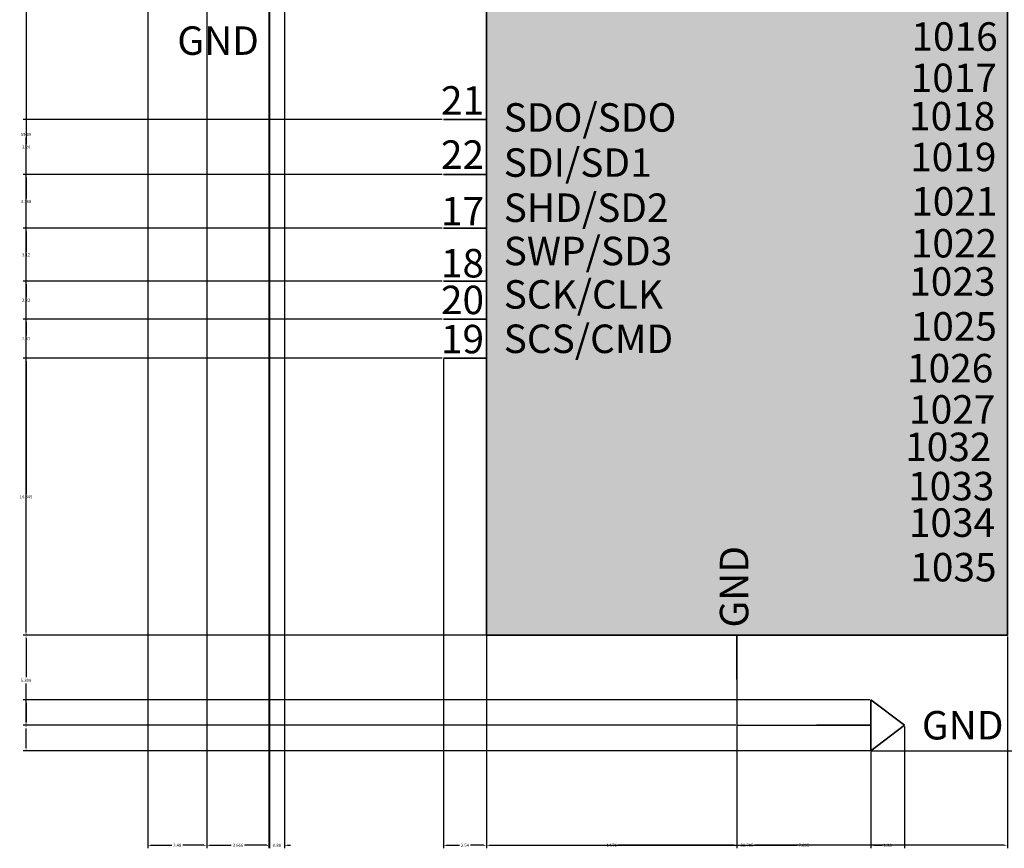
# Model space of a CAD drawing. Units: inches. Extents: x 23 to 132, y 5 to 105.
# Tile 1 of 14: x 23 to 81, y 5 to 54. Entities that reach past the tile are written whole.
import ezdxf

# ---------------------------------------------------------------- set-up
doc = ezdxf.new("R2010")
doc.units = ezdxf.units.IN
doc.header["$MEASUREMENT"] = 0
for name, color, linetype, lineweight in [('A-ANNO-DIMS', 2, 'Continuous', 18), ('E-ANNO-IDEN', 4, 'Continuous', 18), ('E-ANNO-TEXT', 3, 'Continuous', 18), ('E-SYMB', 1, 'Continuous', 35), ('E-SYMB-PATT', 1, 'Continuous', 18), ('E-WIRE', 3, 'Continuous', 25)]:
    doc.layers.add(name, color=color, linetype=linetype, lineweight=lineweight)
doc.styles.get("Standard").update_dxf_attribs({"font": 'arial.ttf'})
doc.dimstyles.get("Standard").update_dxf_attribs({"dimtxt": 0.18, "dimasz": 0.18, "dimexe": 0.18, "dimexo": 0.0625, "dimgap": 0.09, "dimtad": 0, "dimtih": 1, "dimtoh": 1, "dimdec": 4, "dimzin": 0, "dimdsep": 46, "dimtxsty": 'Standard', "dimcen": 0.09, "dimadec": 0, "dimazin": 0, "dimtfac": 1, "dimtdec": 4, "dimtofl": 0, "dimtmove": 0, "dimatfit": 3, "dimfxl": 1, "dimtolj": 1, "dimtzin": 0, "dimarcsym": 0})

# ---------------------------------------------------------------- blocks, each defined once
blk = doc.blocks.new('*D3')
at = {"layer": 'A-ANNO-DIMS', "color": 0, "lineweight": -2, "transparency": 16777216}
for p, q in [((121.409, 99.285), (129.239, 99.285)), ((129.059, 99.105), (129.059, 55.423)), ((129.059, 11.378), (129.059, 55.06)), ((72.981, 11.198), (129.239, 11.198))]:
    blk.add_line(p, q, dxfattribs=at)
at = {"layer": 'A-ANNO-DIMS', "color": 0, "transparency": 16777216}
for points in [[(129.029, 99.105), (129.089, 99.105), (129.059, 99.285)], [(129.029, 11.378), (129.089, 11.378), (129.059, 11.198)]]:
    blk.add_solid(points, dxfattribs=at)
at = {"layer": 'Defpoints', "color": 0, "transparency": 16777216}
for p in [(121.346, 99.285), (129.059, 99.285), (72.919, 11.198)]:
    blk.add_point(p, dxfattribs=at)
at = {"layer": 'A-ANNO-DIMS', "color": 0, "transparency": 16777216, "insert": (129.059, 55.241), "char_height": 0.18, "attachment_point": 5}
blk.add_mtext('\\A1;88.09', dxfattribs=at)
blk = doc.blocks.new('*D4')
at = {"layer": 'A-ANNO-DIMS', "color": 0, "lineweight": -2, "transparency": 16777216}
for p, q in [((50.265, 17.944), (50.265, 5.443)), ((80.969, 17.944), (80.969, 5.443)), ((50.445, 5.623), (65.153, 5.623)), ((80.789, 5.623), (66.081, 5.623))]:
    blk.add_line(p, q, dxfattribs=at)
at = {"layer": 'A-ANNO-DIMS', "color": 0, "transparency": 16777216}
for points in [[(50.445, 5.653), (50.445, 5.593), (50.265, 5.623)], [(80.789, 5.653), (80.789, 5.593), (80.969, 5.623)]]:
    blk.add_solid(points, dxfattribs=at)
at = {"layer": 'Defpoints', "color": 0, "transparency": 16777216}
for p in [(50.265, 18.007), (80.969, 18.007), (80.969, 5.623)]:
    blk.add_point(p, dxfattribs=at)
at = {"layer": 'A-ANNO-DIMS', "color": 0, "transparency": 16777216, "insert": (65.617, 5.623), "char_height": 0.18, "attachment_point": 5}
blk.add_mtext('\\A1;30.705', dxfattribs=at)
blk = doc.blocks.new('*D5')
at = {"layer": 'A-ANNO-DIMS', "color": 0, "lineweight": -2, "transparency": 16777216}
for p, q in [((50.265, 17.944), (50.265, 5.443)), ((65.024, 17.944), (65.024, 5.443)), ((50.445, 5.623), (57.259, 5.623)), ((64.844, 5.623), (58.029, 5.623))]:
    blk.add_line(p, q, dxfattribs=at)
at = {"layer": 'A-ANNO-DIMS', "color": 0, "transparency": 16777216}
for points in [[(50.445, 5.653), (50.445, 5.593), (50.265, 5.623)], [(64.844, 5.653), (64.844, 5.593), (65.024, 5.623)]]:
    blk.add_solid(points, dxfattribs=at)
at = {"layer": 'Defpoints', "color": 0, "transparency": 16777216}
for p in [(50.265, 18.007), (65.024, 18.007), (65.024, 5.623)]:
    blk.add_point(p, dxfattribs=at)
at = {"layer": 'A-ANNO-DIMS', "color": 0, "transparency": 16777216, "insert": (57.644, 5.623), "char_height": 0.18, "attachment_point": 5}
blk.add_mtext('\\A1;14.76', dxfattribs=at)
blk = doc.blocks.new('*D6')
at = {"layer": 'A-ANNO-DIMS', "color": 0, "lineweight": -2, "transparency": 16777216}
for p, q in [((50.202, 77.095), (22.942, 77.095)), ((23.122, 76.915), (23.122, 47.733)), ((23.122, 18.187), (23.122, 47.369)), ((50.202, 18.007), (22.942, 18.007))]:
    blk.add_line(p, q, dxfattribs=at)
at = {"layer": 'A-ANNO-DIMS', "color": 0, "transparency": 16777216}
for points in [[(23.092, 76.915), (23.152, 76.915), (23.122, 77.095)], [(23.092, 18.187), (23.152, 18.187), (23.122, 18.007)]]:
    blk.add_solid(points, dxfattribs=at)
at = {"layer": 'Defpoints', "color": 0, "transparency": 16777216}
for p in [(23.122, 77.095), (50.265, 77.095), (50.265, 18.007)]:
    blk.add_point(p, dxfattribs=at)
at = {"layer": 'A-ANNO-DIMS', "color": 0, "transparency": 16777216, "insert": (23.122, 47.551), "char_height": 0.18, "attachment_point": 5}
blk.add_mtext('\\A1;59.09', dxfattribs=at)
blk = doc.blocks.new('*D8')
at = {"layer": 'A-ANNO-DIMS', "color": 0, "lineweight": -2, "transparency": 16777216}
for p, q in [((64.961, 18.007), (22.942, 18.007)), ((23.122, 17.827), (23.122, 15.534)), ((23.122, 12.878), (23.122, 15.17)), ((64.961, 12.698), (22.942, 12.698))]:
    blk.add_line(p, q, dxfattribs=at)
at = {"layer": 'A-ANNO-DIMS', "color": 0, "transparency": 16777216}
for points in [[(23.092, 17.827), (23.152, 17.827), (23.122, 18.007)], [(23.092, 12.878), (23.152, 12.878), (23.122, 12.698)]]:
    blk.add_solid(points, dxfattribs=at)
at = {"layer": 'Defpoints', "color": 0, "transparency": 16777216}
for p in [(23.122, 18.007), (65.024, 18.007), (65.024, 12.698)]:
    blk.add_point(p, dxfattribs=at)
at = {"layer": 'A-ANNO-DIMS', "color": 0, "transparency": 16777216, "insert": (23.122, 15.352), "char_height": 0.18, "attachment_point": 5}
blk.add_mtext('\\A1;5.308', dxfattribs=at)
blk = doc.blocks.new('*D9')
at = {"layer": 'A-ANNO-DIMS', "color": 0, "lineweight": -2, "transparency": 16777216}
for p, q in [((65.024, 12.636), (65.024, 5.443)), ((72.919, 12.636), (72.919, 5.443)), ((65.204, 5.623), (68.578, 5.623)), ((72.739, 5.623), (69.365, 5.623))]:
    blk.add_line(p, q, dxfattribs=at)
at = {"layer": 'A-ANNO-DIMS', "color": 0, "transparency": 16777216}
for points in [[(65.204, 5.653), (65.204, 5.593), (65.024, 5.623)], [(72.739, 5.653), (72.739, 5.593), (72.919, 5.623)]]:
    blk.add_solid(points, dxfattribs=at)
at = {"layer": 'Defpoints', "color": 0, "transparency": 16777216}
for p in [(65.024, 12.698), (72.919, 12.698), (72.919, 5.623)]:
    blk.add_point(p, dxfattribs=at)
at = {"layer": 'A-ANNO-DIMS', "color": 0, "transparency": 16777216, "insert": (68.971, 5.623), "char_height": 0.18, "attachment_point": 5}
blk.add_mtext('\\A1;7.895', dxfattribs=at)
blk = doc.blocks.new('*D10')
at = {"layer": 'A-ANNO-DIMS', "color": 0, "lineweight": -2, "transparency": 16777216}
for p, q in [((74.903, 12.636), (74.903, 5.443)), ((72.919, 11.136), (72.919, 5.443)), ((73.099, 5.623), (73.595, 5.623)), ((74.723, 5.623), (74.226, 5.623))]:
    blk.add_line(p, q, dxfattribs=at)
at = {"layer": 'A-ANNO-DIMS', "color": 0, "transparency": 16777216}
for points in [[(73.099, 5.653), (73.099, 5.593), (72.919, 5.623)], [(74.723, 5.653), (74.723, 5.593), (74.903, 5.623)]]:
    blk.add_solid(points, dxfattribs=at)
at = {"layer": 'Defpoints', "color": 0, "transparency": 16777216}
for p in [(74.903, 12.698), (72.919, 11.198), (74.903, 5.623)]:
    blk.add_point(p, dxfattribs=at)
at = {"layer": 'A-ANNO-DIMS', "color": 0, "transparency": 16777216, "insert": (73.911, 5.623), "char_height": 0.18, "attachment_point": 5}
blk.add_mtext('\\A1;1.98', dxfattribs=at)
blk = doc.blocks.new('*D11')
at = {"layer": 'A-ANNO-DIMS', "color": 0, "lineweight": -2, "transparency": 16777216}
for p, q in [((72.856, 14.198), (22.942, 14.198)), ((23.122, 14.018), (23.122, 12.88)), ((23.122, 11.378), (23.122, 12.516)), ((72.856, 11.198), (22.942, 11.198))]:
    blk.add_line(p, q, dxfattribs=at)
at = {"layer": 'A-ANNO-DIMS', "color": 0, "transparency": 16777216}
for points in [[(23.092, 14.018), (23.152, 14.018), (23.122, 14.198)], [(23.092, 11.378), (23.152, 11.378), (23.122, 11.198)]]:
    blk.add_solid(points, dxfattribs=at)
at = {"layer": 'Defpoints', "color": 0, "transparency": 16777216}
for p in [(23.122, 14.198), (72.919, 14.198), (72.919, 11.198)]:
    blk.add_point(p, dxfattribs=at)
at = {"layer": 'A-ANNO-DIMS', "color": 0, "transparency": 16777216, "insert": (23.122, 12.698), "char_height": 0.18, "attachment_point": 5}
blk.add_mtext('\\A1;3', dxfattribs=at)
blk = doc.blocks.new('*D13')
at = {"layer": 'A-ANNO-DIMS', "color": 0, "lineweight": -2, "transparency": 16777216}
for p, q in [((47.72, 34.289), (47.72, 5.443)), ((50.265, 34.289), (50.265, 5.443)), ((47.9, 5.623), (48.667, 5.623)), ((50.085, 5.623), (49.317, 5.623))]:
    blk.add_line(p, q, dxfattribs=at)
at = {"layer": 'A-ANNO-DIMS', "color": 0, "transparency": 16777216}
for points in [[(47.9, 5.653), (47.9, 5.593), (47.72, 5.623)], [(50.085, 5.653), (50.085, 5.593), (50.265, 5.623)]]:
    blk.add_solid(points, dxfattribs=at)
at = {"layer": 'Defpoints', "color": 0, "transparency": 16777216}
for p in [(47.72, 34.351), (50.265, 34.351), (50.265, 5.623)]:
    blk.add_point(p, dxfattribs=at)
at = {"layer": 'A-ANNO-DIMS', "color": 0, "transparency": 16777216, "insert": (48.992, 5.623), "char_height": 0.18, "attachment_point": 5}
blk.add_mtext('\\A1;2.54', dxfattribs=at)
blk = doc.blocks.new('*D18')
at = {"layer": 'A-ANNO-DIMS', "color": 0, "lineweight": -2, "transparency": 16777216}
for p, q in [((47.658, 34.351), (22.942, 34.351)), ((23.122, 34.171), (23.122, 26.361)), ((23.122, 18.187), (23.122, 25.997)), ((50.202, 18.007), (22.942, 18.007))]:
    blk.add_line(p, q, dxfattribs=at)
at = {"layer": 'A-ANNO-DIMS', "color": 0, "transparency": 16777216}
for points in [[(23.092, 34.171), (23.152, 34.171), (23.122, 34.351)], [(23.092, 18.187), (23.152, 18.187), (23.122, 18.007)]]:
    blk.add_solid(points, dxfattribs=at)
at = {"layer": 'Defpoints', "color": 0, "transparency": 16777216}
for p in [(23.122, 34.351), (47.72, 34.351), (50.265, 18.007)]:
    blk.add_point(p, dxfattribs=at)
at = {"layer": 'A-ANNO-DIMS', "color": 0, "transparency": 16777216, "insert": (23.122, 26.179), "char_height": 0.18, "attachment_point": 5}
blk.add_mtext('\\A1;16.345', dxfattribs=at)
blk = doc.blocks.new('*D19')
at = {"layer": 'A-ANNO-DIMS', "color": 0, "lineweight": -2, "transparency": 16777216}
for p, q in [((47.658, 36.662), (22.942, 36.662)), ((23.122, 36.482), (23.122, 35.688)), ((23.122, 34.531), (23.122, 35.325)), ((47.658, 34.351), (22.942, 34.351))]:
    blk.add_line(p, q, dxfattribs=at)
at = {"layer": 'A-ANNO-DIMS', "color": 0, "transparency": 16777216}
for points in [[(23.092, 36.482), (23.152, 36.482), (23.122, 36.662)], [(23.092, 34.531), (23.152, 34.531), (23.122, 34.351)]]:
    blk.add_solid(points, dxfattribs=at)
at = {"layer": 'Defpoints', "color": 0, "transparency": 16777216}
for p in [(23.122, 36.662), (47.72, 36.662), (47.72, 34.351)]:
    blk.add_point(p, dxfattribs=at)
at = {"layer": 'A-ANNO-DIMS', "color": 0, "transparency": 16777216, "insert": (23.122, 35.506), "char_height": 0.18, "attachment_point": 5}
blk.add_mtext('\\A1;2.31', dxfattribs=at)
blk = doc.blocks.new('*D20')
at = {"layer": 'A-ANNO-DIMS', "color": 0, "lineweight": -2, "transparency": 16777216}
for p, q in [((47.658, 38.89), (22.942, 38.89)), ((23.122, 38.71), (23.122, 37.958)), ((23.122, 36.842), (23.122, 37.594)), ((47.658, 36.662), (22.942, 36.662))]:
    blk.add_line(p, q, dxfattribs=at)
at = {"layer": 'A-ANNO-DIMS', "color": 0, "transparency": 16777216}
for points in [[(23.092, 38.71), (23.152, 38.71), (23.122, 38.89)], [(23.092, 36.842), (23.152, 36.842), (23.122, 36.662)]]:
    blk.add_solid(points, dxfattribs=at)
at = {"layer": 'Defpoints', "color": 0, "transparency": 16777216}
for p in [(23.122, 38.89), (47.72, 38.89), (47.72, 36.662)]:
    blk.add_point(p, dxfattribs=at)
at = {"layer": 'A-ANNO-DIMS', "color": 0, "transparency": 16777216, "insert": (23.122, 37.776), "char_height": 0.18, "attachment_point": 5}
blk.add_mtext('\\A1;2.23', dxfattribs=at)
blk = doc.blocks.new('*D21')
at = {"layer": 'A-ANNO-DIMS', "color": 0, "lineweight": -2, "transparency": 16777216}
for p, q in [((47.658, 42.013), (22.942, 42.013)), ((23.122, 41.833), (23.122, 40.634)), ((23.122, 39.07), (23.122, 40.27)), ((47.658, 38.89), (22.942, 38.89))]:
    blk.add_line(p, q, dxfattribs=at)
at = {"layer": 'A-ANNO-DIMS', "color": 0, "transparency": 16777216}
for points in [[(23.092, 41.833), (23.152, 41.833), (23.122, 42.013)], [(23.092, 39.07), (23.152, 39.07), (23.122, 38.89)]]:
    blk.add_solid(points, dxfattribs=at)
at = {"layer": 'Defpoints', "color": 0, "transparency": 16777216}
for p in [(23.122, 42.013), (47.72, 42.013), (47.72, 38.89)]:
    blk.add_point(p, dxfattribs=at)
at = {"layer": 'A-ANNO-DIMS', "color": 0, "transparency": 16777216, "insert": (23.122, 40.452), "char_height": 0.18, "attachment_point": 5}
blk.add_mtext('\\A1;3.12', dxfattribs=at)
blk = doc.blocks.new('*D22')
at = {"layer": 'A-ANNO-DIMS', "color": 0, "lineweight": -2, "transparency": 16777216}
for p, q in [((47.658, 45.181), (22.942, 45.181)), ((23.122, 45.001), (23.122, 43.779)), ((23.122, 42.193), (23.122, 43.415)), ((47.658, 42.013), (22.942, 42.013))]:
    blk.add_line(p, q, dxfattribs=at)
at = {"layer": 'A-ANNO-DIMS', "color": 0, "transparency": 16777216}
for points in [[(23.092, 45.001), (23.152, 45.001), (23.122, 45.181)], [(23.092, 42.193), (23.152, 42.193), (23.122, 42.013)]]:
    blk.add_solid(points, dxfattribs=at)
at = {"layer": 'Defpoints', "color": 0, "transparency": 16777216}
for p in [(23.122, 45.181), (47.72, 45.181), (47.72, 42.013)]:
    blk.add_point(p, dxfattribs=at)
at = {"layer": 'A-ANNO-DIMS', "color": 0, "transparency": 16777216, "insert": (23.122, 43.597), "char_height": 0.18, "attachment_point": 5}
blk.add_mtext('\\A1;3.168', dxfattribs=at)
blk = doc.blocks.new('*D23')
at = {"layer": 'A-ANNO-DIMS', "color": 0, "lineweight": -2, "transparency": 16777216}
for p, q in [((47.658, 48.422), (22.942, 48.422)), ((23.122, 48.242), (23.122, 46.984)), ((23.122, 45.361), (23.122, 46.62)), ((47.658, 45.181), (22.942, 45.181))]:
    blk.add_line(p, q, dxfattribs=at)
at = {"layer": 'A-ANNO-DIMS', "color": 0, "transparency": 16777216}
for points in [[(23.092, 48.242), (23.152, 48.242), (23.122, 48.422)], [(23.092, 45.361), (23.152, 45.361), (23.122, 45.181)]]:
    blk.add_solid(points, dxfattribs=at)
at = {"layer": 'Defpoints', "color": 0, "transparency": 16777216}
for p in [(23.122, 48.422), (47.72, 48.422), (47.72, 45.181)]:
    blk.add_point(p, dxfattribs=at)
at = {"layer": 'A-ANNO-DIMS', "color": 0, "transparency": 16777216, "insert": (23.122, 46.802), "char_height": 0.18, "attachment_point": 5}
blk.add_mtext('\\A1;3.24', dxfattribs=at)
blk = doc.blocks.new('*D55')
at = {"layer": 'A-ANNO-DIMS', "color": 0, "lineweight": -2, "transparency": 16777216}
for p, q in [((30.295, 59.913), (30.295, 5.443)), ((33.776, 59.889), (33.776, 5.443)), ((30.475, 5.623), (31.712, 5.623)), ((33.596, 5.623), (32.359, 5.623))]:
    blk.add_line(p, q, dxfattribs=at)
at = {"layer": 'A-ANNO-DIMS', "color": 0, "transparency": 16777216}
for points in [[(30.475, 5.653), (30.475, 5.593), (30.295, 5.623)], [(33.596, 5.653), (33.596, 5.593), (33.776, 5.623)]]:
    blk.add_solid(points, dxfattribs=at)
at = {"layer": 'Defpoints', "color": 0, "transparency": 16777216}
for p in [(30.295, 59.975), (33.776, 59.951), (33.776, 5.623)]:
    blk.add_point(p, dxfattribs=at)
at = {"layer": 'A-ANNO-DIMS', "color": 0, "transparency": 16777216, "insert": (32.036, 5.623), "char_height": 0.18, "attachment_point": 5}
blk.add_mtext('\\A1;3.48', dxfattribs=at)
blk = doc.blocks.new('*D56')
at = {"layer": 'A-ANNO-DIMS', "color": 0, "lineweight": -2, "transparency": 16777216}
for p, q in [((33.776, 59.889), (33.776, 5.443)), ((37.442, 59.913), (37.442, 5.443)), ((33.956, 5.623), (35.215, 5.623)), ((37.262, 5.623), (36.002, 5.623))]:
    blk.add_line(p, q, dxfattribs=at)
at = {"layer": 'A-ANNO-DIMS', "color": 0, "transparency": 16777216}
for points in [[(33.956, 5.653), (33.956, 5.593), (33.776, 5.623)], [(37.262, 5.653), (37.262, 5.593), (37.442, 5.623)]]:
    blk.add_solid(points, dxfattribs=at)
at = {"layer": 'Defpoints', "color": 0, "transparency": 16777216}
for p in [(33.776, 59.951), (37.442, 59.975), (37.442, 5.623)]:
    blk.add_point(p, dxfattribs=at)
at = {"layer": 'A-ANNO-DIMS', "color": 0, "transparency": 16777216, "insert": (35.609, 5.623), "char_height": 0.18, "attachment_point": 5}
blk.add_mtext('\\A1;3.666', dxfattribs=at)
blk = doc.blocks.new('*D66')
at = {"layer": 'A-ANNO-DIMS', "color": 0, "lineweight": -2, "transparency": 16777216}
for p, q in [((37.473, 64.488), (37.473, 5.443)), ((38.351, 64.418), (38.351, 5.443)), ((37.293, 5.623), (37.113, 5.623)), ((38.531, 5.623), (38.711, 5.623))]:
    blk.add_line(p, q, dxfattribs=at)
at = {"layer": 'A-ANNO-DIMS', "color": 0, "transparency": 16777216}
for points in [[(37.293, 5.653), (37.293, 5.593), (37.473, 5.623)], [(38.531, 5.653), (38.531, 5.593), (38.351, 5.623)]]:
    blk.add_solid(points, dxfattribs=at)
at = {"layer": 'Defpoints', "color": 0, "transparency": 16777216}
for p in [(37.473, 64.551), (38.351, 64.48), (38.351, 5.623)]:
    blk.add_point(p, dxfattribs=at)
at = {"layer": 'A-ANNO-DIMS', "color": 0, "transparency": 16777216, "insert": (37.912, 5.623), "char_height": 0.18, "attachment_point": 5}
blk.add_mtext('\\A1;0.88', dxfattribs=at)

msp = doc.modelspace()

# ---------------------------------------------------------------- hatches: boundary and pattern name
at = {"layer": 'E-SYMB-PATT'}
h = msp.add_hatch(color=256, dxfattribs=at)
h.dxf.hatch_style = 1
h.paths.add_polyline_path([(80.9692, 77.095), (50.2646, 77.095), (50.2646, 18.0066), (80.9692, 18.0066)])

# ---------------------------------------------------------------- linework, layer by layer
at = {"layer": 'E-SYMB'}
for p, q in [((47.7202, 48.4225), (50.2646, 48.4225)), ((47.7202, 45.1811), (50.2646, 45.1811)), ((47.7202, 42.0128), (50.2646, 42.0128)), ((47.7202, 38.8905), (50.2646, 38.8905)), ((47.7202, 36.6618), (50.2646, 36.6618)), ((47.7202, 34.3512), (50.2646, 34.3512)), ((65.0236, 18.0066), (65.0236, 15.3982)), ((72.9188, 12.6983), (72.9188, 14.1983)), ((72.9188, 14.1983), (74.9031, 12.6983)), ((69.71, 12.6983), (72.9188, 12.6983)), ((72.9188, 12.6983), (72.9188, 11.1983)), ((72.9188, 11.1983), (74.9031, 12.6983))]:
    msp.add_line(p, q, dxfattribs=at)
msp.add_lwpolyline([(50.2646, 77.095), (80.9692, 77.095), (80.9692, 18.0066), (50.2646, 18.0066)], close=True, dxfattribs=at)
at = {"layer": 'E-WIRE'}
for p, q in [((65.0236, 15.3982), (65.0236, 12.6983)), ((65.0236, 12.6983), (69.71, 12.6983))]:
    msp.add_line(p, q, dxfattribs=at)

# ---------------------------------------------------------------- texts
at = {"layer": 'E-ANNO-IDEN'}
for p in [(32.0372, 52.2438), (75.9297, 11.8627)]:
    msp.add_text('GND', height=1.67943, dxfattribs=at).set_placement(p)
msp.add_text('GND', height=1.67943, rotation=90, dxfattribs=at).set_placement((65.6976, 18.4654))
at = {"layer": 'E-ANNO-TEXT'}
for s, p in [('1016', (75.3118, 52.4857)), ('1017', (75.268, 50.0483)), ('21', (47.5772, 48.717)), ('SDO/SDO', (51.2785, 47.7127)), ('1018', (75.1713, 47.788)), ('22', (47.5772, 45.5201)), ('1019', (75.2359, 45.3821)), ('SDI/SD1', (51.2785, 45.0501)), ('SHD/SD2', (51.2785, 42.3896)), ('1021', (75.2982, 42.764)), ('17', (47.5772, 42.1874)), ('1022', (75.279, 40.2939)), ('SWP/SD3', (51.2785, 39.8347)), ('18', (47.5772, 39.1156)), ('1023', (75.1827, 38.0386)), ('SCK/CLK', (51.2785, 37.2749)), ('20', (47.5772, 36.9496)), ('1025', (75.2665, 35.3895)), ('19', (47.5772, 34.639)), ('SCS/CMD', (51.2785, 34.6576)), ('1026', (75.0517, 32.925)), ('1027', (75.1733, 30.4918)), ('1032', (74.9426, 28.282)), ('1033', (75.1177, 25.9659)), ('1034', (75.1611, 23.8143)), ('1035', (75.2464, 21.1859))]:
    msp.add_text(s, height=1.67943, dxfattribs=at).set_placement(p)

# ---------------------------------------------------------------- dimensions: what is measured, and where the dimension line sits
at = {"layer": 'A-ANNO-DIMS'}
for base, p1, p2, override, picture, middle in [((129.0589, 99.2846), (72.9188, 11.1983), (121.3461, 99.2846), {"dimdec": 2, "dimlfac": 1, "dimrnd": 0, "dimzin": 0, "dimdsep": 46, "dimlunit": 2}, '*D3', (129.0589, 55.2415)), ((23.1215, 77.095), (50.2646, 18.0066), (50.2646, 77.095), {"dimdec": 2, "dimlfac": 1, "dimrnd": 0, "dimzin": 0, "dimdsep": 46, "dimlunit": 2}, '*D6', (23.1215, 47.5508)), ((23.1215, 48.4225), (47.7202, 45.1811), (47.7202, 48.4225), {"dimdec": 2, "dimlfac": 1, "dimrnd": 0, "dimzin": 0, "dimdsep": 46, "dimlunit": 2}, '*D23', (23.1215, 46.8018)), ((23.1215, 45.1811), (47.7202, 42.0128), (47.7202, 45.1811), {"dimdec": 3, "dimlfac": 1, "dimrnd": 0, "dimzin": 0, "dimdsep": 46, "dimlunit": 2}, '*D22', (23.1215, 43.5969)), ((23.1215, 42.0128), (47.7202, 38.8905), (47.7202, 42.0128), {"dimdec": 2, "dimlfac": 1, "dimrnd": 0, "dimzin": 0, "dimdsep": 46, "dimlunit": 2}, '*D21', (23.1215, 40.4516)), ((23.1215, 38.8905), (47.7202, 36.6618), (47.7202, 38.8905), {"dimdec": 2, "dimlfac": 1, "dimrnd": 0, "dimzin": 0, "dimdsep": 46, "dimlunit": 2}, '*D20', (23.1215, 37.7761)), ((23.1215, 36.6618), (47.7202, 34.3512), (47.7202, 36.6618), {"dimdec": 2, "dimlfac": 1, "dimrnd": 0, "dimzin": 0, "dimdsep": 46, "dimlunit": 2}, '*D19', (23.1215, 35.5065)), ((23.1215, 34.3512), (50.2646, 18.0066), (47.7202, 34.3512), {"dimdec": 3, "dimlfac": 1, "dimrnd": 0, "dimzin": 0, "dimdsep": 46, "dimlunit": 2}, '*D18', (23.1215, 26.1789)), ((23.1215, 18.0066), (65.0236, 12.6983), (65.0236, 18.0066), {"dimdec": 3, "dimlfac": 1, "dimrnd": 0, "dimzin": 0, "dimdsep": 46, "dimlunit": 2}, '*D8', (23.1215, 15.3524)), ((23.1215, 14.1983), (72.9188, 11.1983), (72.9188, 14.1983), {"dimdec": 0, "dimlfac": 1, "dimrnd": 0, "dimzin": 0, "dimdsep": 46, "dimlunit": 2}, '*D11', (23.1215, 12.6983))]:
    dim = msp.add_linear_dim(base=base, p1=p1, p2=p2, angle=90, dimstyle='Standard', override=override, dxfattribs=at)
    dim.commit()
    dim.dimension.update_dxf_attribs({"geometry": picture, "text_midpoint": middle})
for base, p1, p2, override, picture, middle in [((38.3512, 5.6233), (37.473, 64.5505), (38.3512, 64.4801), {"dimdec": 2, "dimlfac": 1, "dimrnd": 0, "dimzin": 0, "dimdsep": 46, "dimlunit": 2}, '*D66', (37.9121, 5.6233)), ((33.7757, 5.6233), (30.2954, 59.9755), (33.7757, 59.951), {"dimdec": 2, "dimlfac": 1, "dimrnd": 0, "dimzin": 0, "dimdsep": 46, "dimlunit": 2}, '*D55', (32.0356, 5.6233)), ((37.442, 5.6233), (33.7757, 59.951), (37.442, 59.9755), {"dimdec": 3, "dimlfac": 1, "dimrnd": 0, "dimzin": 0, "dimdsep": 46, "dimlunit": 2}, '*D56', (35.6089, 5.6233)), ((50.2646, 5.6233), (47.7202, 34.3512), (50.2646, 34.3512), {"dimdec": 2, "dimlfac": 1, "dimrnd": 0, "dimzin": 0, "dimdsep": 46, "dimlunit": 2}, '*D13', (48.9924, 5.6233)), ((80.9692, 5.6233), (50.2646, 18.0066), (80.9692, 18.0066), {"dimdec": 3, "dimlfac": 1, "dimrnd": 0, "dimzin": 0, "dimdsep": 46, "dimlunit": 2}, '*D4', (65.6169, 5.6233)), ((65.0236, 5.6233), (50.2646, 18.0066), (65.0236, 18.0066), {"dimdec": 2, "dimlfac": 1, "dimrnd": 0, "dimzin": 0, "dimdsep": 46, "dimlunit": 2}, '*D5', (57.6441, 5.6233)), ((72.9188, 5.6233), (65.0236, 12.6983), (72.9188, 12.6983), {"dimdec": 3, "dimlfac": 1, "dimrnd": 0, "dimzin": 0, "dimdsep": 46, "dimlunit": 2}, '*D9', (68.9712, 5.6233)), ((74.9031, 5.6233), (72.9188, 11.1983), (74.9031, 12.6983), {"dimdec": 2, "dimlfac": 1, "dimrnd": 0, "dimzin": 0, "dimdsep": 46, "dimlunit": 2}, '*D10', (73.9109, 5.6233))]:
    dim = msp.add_linear_dim(base=base, p1=p1, p2=p2, dimstyle='Standard', override=override, dxfattribs=at)
    dim.commit()
    dim.dimension.update_dxf_attribs({"geometry": picture, "text_midpoint": middle})

doc.saveas('drawing.dxf')
